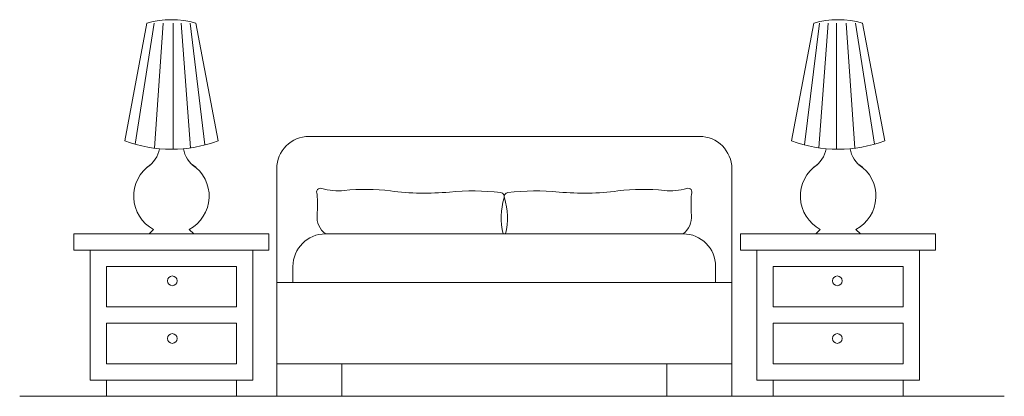
# Model space of a CAD drawing. Units: inches. Extents: x 1994 to 3075, y 3517 to 3950.
# Tile 32 of 58: x 1994.6375 to 1994.7567, y 3553.6033 to 3553.6489. Entities that reach past the tile are written whole.
import ezdxf

# ---------------------------------------------------------------- set-up
doc = ezdxf.new("R2010")
doc.units = ezdxf.units.IN
doc.layers.add('A-FURN-REFR', color=8, linetype='Continuous', lineweight=13)

msp = doc.modelspace()

# ---------------------------------------------------------------- linework, layer by layer
at = {"layer": 'A-FURN-REFR', "ltscale": 2}
for p, q in [((1994.650198191188, 3553.634267887672), (1994.652894564834, 3553.648504740526)), ((1994.653751479282, 3553.648504740526), (1994.651452910123, 3553.633851910284)), ((1994.654859422462, 3553.648504740526), (1994.653820033808, 3553.633364448499)), ((1994.656055256143, 3553.648504740526), (1994.656055256143, 3553.63323617785)), ((1994.657050637775, 3553.648504740526), (1994.658181851277, 3553.633405717129)), ((1994.658106288641, 3553.648504740526), (1994.65991548662, 3553.633760249959)), ((1994.661504080468, 3553.634267887672), (1994.658807706821, 3553.648504740526)), ((1994.730933177028, 3553.634267887672), (1994.733629550674, 3553.648504740526)), ((1994.734330968855, 3553.648504740526), (1994.732521770876, 3553.633760249959)), ((1994.735386619721, 3553.648504740526), (1994.734255406219, 3553.633405717129)), ((1994.736382001353, 3553.648504740526), (1994.736382001353, 3553.63323617785)), ((1994.737577835033, 3553.648504740526), (1994.738617223688, 3553.633364448499)), ((1994.738685778214, 3553.648504740526), (1994.740984347373, 3553.633851910284)), ((1994.742239066308, 3553.634267887672), (1994.739542692661, 3553.648504740526)), ((1994.672539170393, 3553.634790093627), (1994.719783264881, 3553.634790093627)), ((1994.668602162519, 3553.630853085753), (1994.668602162519, 3553.603294030634)), ((1994.723720272755, 3553.603294030634), (1994.723720272755, 3553.630853085753)), ((1994.644040112206, 3553.622979070004), (1994.644040112206, 3553.621010566067)), ((1994.66766215945, 3553.622979070004), (1994.644040112206, 3553.622979070004)), ((1994.653154762181, 3553.622979070004), (1994.653695074031, 3553.623519381853)), ((1994.658547509475, 3553.622979070004), (1994.653154762181, 3553.622979070004)), ((1994.658547509475, 3553.622979070004), (1994.658007197625, 3553.623519381853)), ((1994.66766215945, 3553.621010566067), (1994.66766215945, 3553.622979070004)), ((1994.717814760944, 3553.622979070004), (1994.67450767433, 3553.622979070004)), ((1994.724775098046, 3553.621010566067), (1994.724775098046, 3553.622979070004)), ((1994.724775098046, 3553.622979070004), (1994.74839714529, 3553.622979070004)), ((1994.733889748021, 3553.622979070004), (1994.734430059871, 3553.623519381853)), ((1994.733889748021, 3553.622979070004), (1994.739282495315, 3553.622979070004)), ((1994.739282495315, 3553.622979070004), (1994.738742183465, 3553.623519381853)), ((1994.74839714529, 3553.622979070004), (1994.74839714529, 3553.621010566067)), ((1994.644040112206, 3553.621010566067), (1994.66766215945, 3553.621010566067)), ((1994.646008616143, 3553.605262534571), (1994.646008616143, 3553.621010566067)), ((1994.665693655513, 3553.621010566067), (1994.665693655513, 3553.605262534571)), ((1994.74839714529, 3553.621010566067), (1994.724775098046, 3553.621010566067)), ((1994.726743601983, 3553.621010566067), (1994.726743601983, 3553.605262534571)), ((1994.746428641353, 3553.605262534571), (1994.746428641353, 3553.621010566067)), ((1994.64797712008, 3553.614120802288), (1994.64797712008, 3553.61904206213)), ((1994.64797712008, 3553.61904206213), (1994.663725151576, 3553.61904206213)), ((1994.663725151576, 3553.61904206213), (1994.663725151576, 3553.614120802288)), ((1994.670570666456, 3553.617073558193), (1994.670570666456, 3553.61904206213)), ((1994.721751768818, 3553.617073558193), (1994.721751768818, 3553.61904206213)), ((1994.72871210592, 3553.61904206213), (1994.72871210592, 3553.614120802288)), ((1994.744460137416, 3553.61904206213), (1994.72871210592, 3553.61904206213)), ((1994.744460137416, 3553.614120802288), (1994.744460137416, 3553.61904206213)), ((1994.668602162519, 3553.617073558193), (1994.723720272755, 3553.617073558193)), ((1994.64797712008, 3553.614120802288), (1994.663725151576, 3553.614120802288)), ((1994.744460137416, 3553.614120802288), (1994.72871210592, 3553.614120802288)), ((1994.663725151576, 3553.612152298351), (1994.64797712008, 3553.612152298351)), ((1994.64797712008, 3553.607231038508), (1994.64797712008, 3553.612152298351)), ((1994.663725151576, 3553.612152298351), (1994.663725151576, 3553.607231038508)), ((1994.72871210592, 3553.612152298351), (1994.72871210592, 3553.607231038508)), ((1994.72871210592, 3553.612152298351), (1994.744460137416, 3553.612152298351)), ((1994.744460137416, 3553.607231038508), (1994.744460137416, 3553.612152298351)), ((1994.663725151576, 3553.607231038508), (1994.64797712008, 3553.607231038508)), ((1994.668602162519, 3553.607231038508), (1994.723720272755, 3553.607231038508)), ((1994.676476178267, 3553.607231038508), (1994.676476178267, 3553.603294030634)), ((1994.715846257007, 3553.603294030634), (1994.715846257007, 3553.607231038508)), ((1994.72871210592, 3553.607231038508), (1994.744460137416, 3553.607231038508)), ((1994.665693655513, 3553.605262534571), (1994.646008616143, 3553.605262534571)), ((1994.64797712008, 3553.603294030634), (1994.64797712008, 3553.605262534571)), ((1994.663725151576, 3553.605262534571), (1994.663725151576, 3553.603294030634)), ((1994.726743601983, 3553.605262534571), (1994.746428641353, 3553.605262534571)), ((1994.72871210592, 3553.605262534571), (1994.72871210592, 3553.603294030634)), ((1994.744460137416, 3553.603294030634), (1994.744460137416, 3553.605262534571)), ((1994.663725151576, 3553.603294030634), (1994.64797712008, 3553.603294030634)), ((1994.668602162519, 3553.603294030634), (1994.676476178267, 3553.603294030634)), ((1994.715846257007, 3553.603294030634), (1994.723720272755, 3553.603294030634)), ((1994.72871210592, 3553.603294030634), (1994.744460137416, 3553.603294030634))]:
    msp.add_line(p, q, dxfattribs=at)
at = {"layer": 'A-FURN-REFR'}
msp.add_line((1994.756710685442, 3553.603294030634), (1994.63747988638, 3553.603294030634), dxfattribs=at)
at = {"layer": 'A-FURN-REFR', "ltscale": 2}
for points in [[(1994.650198191188, 3553.634267887672, 0.1827389611657951), (1994.661504080468, 3553.634267887672, 0.5486822924550565)], [(1994.742239066308, 3553.634267887672, -0.1827389611657951), (1994.730933177028, 3553.634267887672, -0.5486822924550565)], [(1994.696020526266, 3553.622979070004, -0.1353662691233677), (1994.69614169022, 3553.627348148405, 0.4688378584060677), (1994.695725183871, 3553.627983879014, 0.0519081028429589), (1994.689529651916, 3553.628047452075, -0.0557006724553551), (1994.682396980675, 3553.628174598197, 0.0589705110073461), (1994.676774144952, 3553.628238171258, -0.1004118058571634), (1994.674066853678, 3553.628492463501, 0.6684064296708754), (1994.673494157447, 3553.627793159832, -0.0436722497868855), (1994.673494157447, 3553.625250237396, 0.2590858381004083), (1994.67450767433, 3553.622979070004, 0.2980829464224009)], [(1994.696301909008, 3553.622979070004, 0.1353662691233677), (1994.696180745054, 3553.627348148405, -0.4688378584060677), (1994.696597251403, 3553.627983879014, -0.0519081028429589), (1994.702792783358, 3553.628047452075, 0.0557006724553551), (1994.709925454599, 3553.628174598197, -0.0589705110073461), (1994.715548290322, 3553.628238171258, 0.1004118058571634), (1994.718255581596, 3553.628492463501, -0.6684064296708754), (1994.718828277827, 3553.627793159832, 0.0436722497868855), (1994.718828277827, 3553.625250237396, -0.2590858381004083), (1994.717814760944, 3553.622979070004, -0.2980829464224009)]]:
    msp.add_lwpolyline(points, format="xyb", dxfattribs=at)
for centre in [(1994.655954229057, 3553.617288098165), (1994.736483028438, 3553.617288098165), (1994.655954229057, 3553.610299998803), (1994.736483028438, 3553.610299998803)]:
    msp.add_circle(centre, 0.0005905511811024, dxfattribs=at)
for centre, radius, start, end in [((1994.655851135828, 3553.638452583577), 0.0104779373627493, 73.61017510197637, 106.3898248980236), ((1994.736586121668, 3553.638452583577), 0.0104779373627493, 73.61017510197637, 106.3898248980236), ((1994.672539170393, 3553.630853085753), 0.0039370078740157, 90, 180), ((1994.719783264881, 3553.630853085753), 0.0039370078740157, 0, 90), ((1994.651145668373, 3553.633829683717), 0.0032922334161267, 302.2864548273144, 350.7647725220839), ((1994.660556603283, 3553.633829683717), 0.0032922334161267, 189.2352274779161, 237.7135451726856), ((1994.731880654213, 3553.633829683717), 0.0032922334161267, 302.2864548273144, 350.7647725220839), ((1994.741291589123, 3553.633829683717), 0.0032922334161267, 189.2352274779161, 237.7135451726856), ((1994.655851135828, 3553.627551003209), 0.0045719332043748, 123.5652568840551, 241.8626735144181), ((1994.655851135828, 3553.627551003209), 0.0045719332043748, 298.1373264855819, 56.4347431159449), ((1994.736586121668, 3553.627551003209), 0.0045719332043748, 123.5652568840551, 241.8626735144181), ((1994.736586121668, 3553.627551003209), 0.0045719332043748, 298.1373264855819, 56.4347431159449), ((1994.67450767433, 3553.61904206213), 0.0039370078740157, 90, 180), ((1994.717814760944, 3553.61904206213), 0.0039370078740157, 0, 90)]:
    msp.add_arc(centre, radius, start, end, dxfattribs=at)

doc.saveas('drawing.dxf')
